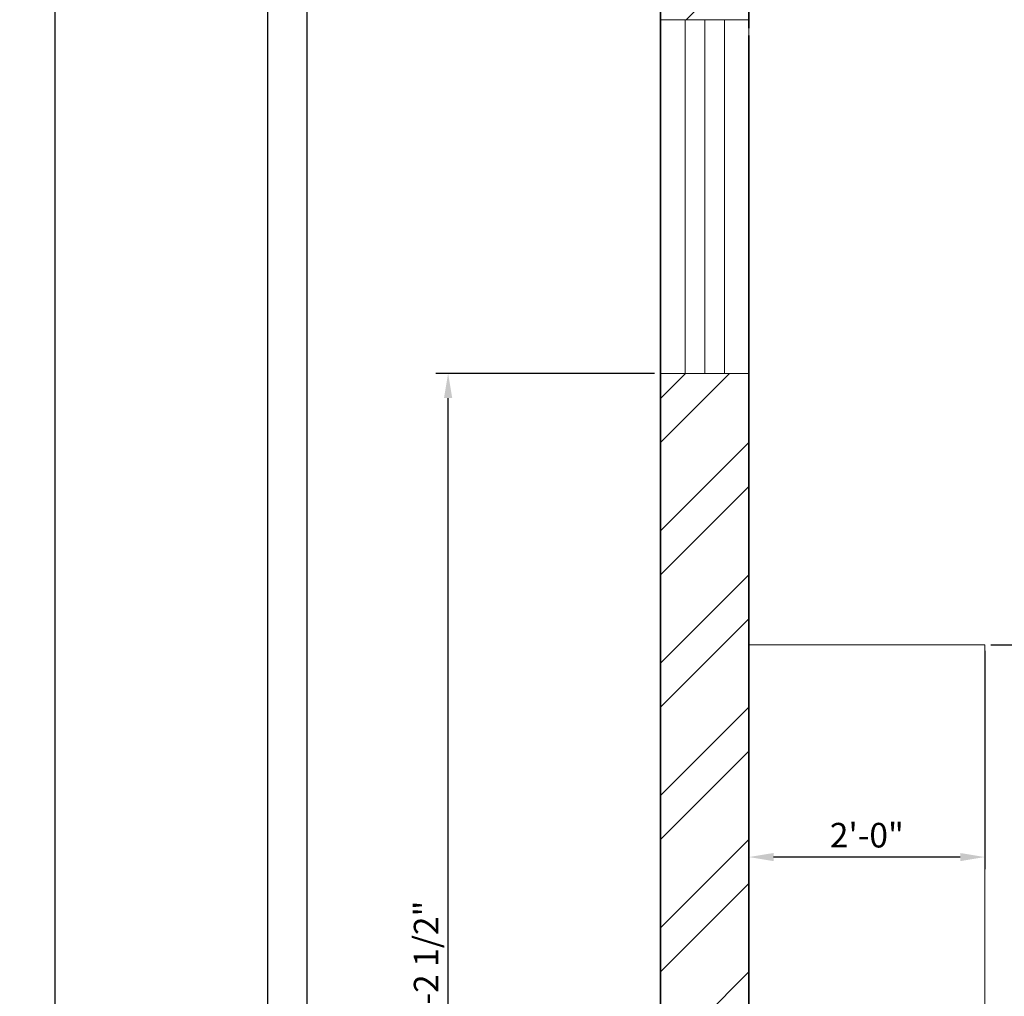
# Model space of a CAD drawing. Units: inches. Extents: x -138 to 270, y 8284 to 8764.
# Tile 2 of 10: x -138 to -38, y 8406 to 8506. Entities that reach past the tile are written whole.
import ezdxf

# ---------------------------------------------------------------- set-up
doc = ezdxf.new("R2010")
doc.units = ezdxf.units.IN
for name, color, linetype, lineweight in [('A-ANNO-DIMS', 2, 'Continuous', 18), ('A-FLOR-CASE', 9, 'Continuous', 18), ('C-PROP', 7, 'Continuous', 25), ('WALL', 8, 'Continuous', 35), ('WINDOW', 151, 'Continuous', 15)]:
    doc.layers.add(name, color=color, linetype=linetype, lineweight=lineweight)
doc.layers.add('A-WALL-PATT', color=32, linetype='Continuous', lineweight=9, true_color=0xbc761a)
doc.styles.get("Standard").update_dxf_attribs({"font": 'arial.ttf'})
doc.dimstyles.new('ISO-25', dxfattribs={"dimtxt": 2.5, "dimasz": 2.5, "dimexe": 1.25, "dimexo": 0.625, "dimtad": 1, "dimdec": 0, "dimlunit": 3, "dimtxsty": 'Standard', "dimcen": 2.5, "dimadec": 0, "dimazin": 0, "dimtfac": 1, "dimtdec": 0, "dimtmove": 0, "dimatfit": 3, "dimfxl": 1, "dimarcsym": 0})

# ---------------------------------------------------------------- blocks, each defined once
blk = doc.blocks.new('WINDOW-36IN')
for p, q in [((0, 6.5), (36, 6.5)), ((0, 4.5), (36, 4.5)), ((0, 2.5), (36, 2.5))]:
    blk.add_line(p, q)
blk.add_lwpolyline([(0, 0), (36, 0), (36, 9), (0, 9)], close=True)
blk = doc.blocks.new('*D52')
at = {"layer": 'A-ANNO-DIMS', "color": 0, "lineweight": -2, "transparency": 16777216}
for p, q in [((-113.55, 8739.24), (-135.79, 8739.24)), ((-134.54, 8309.74), (-134.54, 8736.74)), ((-113.55, 8307.24), (-135.79, 8307.24))]:
    blk.add_line(p, q, dxfattribs=at)
at = {"layer": 'A-ANNO-DIMS', "color": 0, "transparency": 16777216}
for points in [[(-134.96, 8736.74), (-134.12, 8736.74), (-134.54, 8739.24)], [(-134.96, 8309.74), (-134.12, 8309.74), (-134.54, 8307.24)]]:
    blk.add_solid(points, dxfattribs=at)
at = {"layer": 'Defpoints', "color": 0, "transparency": 16777216}
for p in [(-134.54, 8739.24), (-112.92, 8739.24), (-112.92, 8307.24)]:
    blk.add_point(p, dxfattribs=at)
at = {"layer": 'A-ANNO-DIMS', "color": 0, "transparency": 16777216, "insert": (-136.44, 8523.24), "char_height": 2.5, "attachment_point": 5, "rotation": 90}
blk.add_mtext('36\'-0"', dxfattribs=at)
blk = doc.blocks.new('*D64')
at = {"layer": 'A-ANNO-DIMS', "color": 0, "lineweight": -2, "transparency": 16777216}
for p, q in [((-73.55, 8469.84), (-95.79, 8469.84)), ((-94.54, 8349.74), (-94.54, 8467.34)), ((-73.55, 8347.24), (-95.79, 8347.24))]:
    blk.add_line(p, q, dxfattribs=at)
at = {"layer": 'A-ANNO-DIMS', "color": 0, "transparency": 16777216}
for points in [[(-94.96, 8467.34), (-94.12, 8467.34), (-94.54, 8469.84)], [(-94.96, 8349.74), (-94.12, 8349.74), (-94.54, 8347.24)]]:
    blk.add_solid(points, dxfattribs=at)
at = {"layer": 'Defpoints', "color": 0, "transparency": 16777216}
for p in [(-94.54, 8469.84), (-72.92, 8469.84), (-72.92, 8347.24)]:
    blk.add_point(p, dxfattribs=at)
at = {"layer": 'A-ANNO-DIMS', "color": 0, "transparency": 16777216, "insert": (-96.46, 8408.54), "char_height": 2.5, "attachment_point": 5, "rotation": 90}
blk.add_mtext('10\'-2 1/2"', dxfattribs=at)
blk = doc.blocks.new('*D73')
at = {"layer": 'A-ANNO-DIMS', "color": 0, "lineweight": -2, "transparency": 16777216}
for p, q in [((-63.92, 8441.62), (-63.92, 8419.38)), ((-39.92, 8441.62), (-39.92, 8419.38)), ((-42.42, 8420.63), (-61.42, 8420.63))]:
    blk.add_line(p, q, dxfattribs=at)
at = {"layer": 'A-ANNO-DIMS', "color": 0, "transparency": 16777216}
for points in [[(-61.42, 8421.04), (-61.42, 8420.21), (-63.92, 8420.63)], [(-42.42, 8421.04), (-42.42, 8420.21), (-39.92, 8420.63)]]:
    blk.add_solid(points, dxfattribs=at)
at = {"layer": 'Defpoints', "color": 0, "transparency": 16777216}
for p in [(-63.92, 8442.24), (-39.92, 8442.24), (-63.92, 8420.63)]:
    blk.add_point(p, dxfattribs=at)
at = {"layer": 'A-ANNO-DIMS', "color": 0, "transparency": 16777216, "insert": (-51.92, 8422.53), "char_height": 2.5, "attachment_point": 5}
blk.add_mtext('2\'-0"', dxfattribs=at)
blk = doc.blocks.new('*D74')
at = {"layer": 'A-ANNO-DIMS', "color": 0, "lineweight": -2, "transparency": 16777216}
for p, q in [((-39.3, 8442.24), (-17.06, 8442.24)), ((-18.31, 8439.74), (-18.31, 8382.74)), ((-39.3, 8380.24), (-17.06, 8380.24))]:
    blk.add_line(p, q, dxfattribs=at)
at = {"layer": 'A-ANNO-DIMS', "color": 0, "transparency": 16777216}
for points in [[(-18.73, 8439.74), (-17.89, 8439.74), (-18.31, 8442.24)], [(-18.73, 8382.74), (-17.89, 8382.74), (-18.31, 8380.24)]]:
    blk.add_solid(points, dxfattribs=at)
at = {"layer": 'Defpoints', "color": 0, "transparency": 16777216}
for p in [(-39.92, 8442.24), (-39.92, 8380.24), (-18.31, 8380.24)]:
    blk.add_point(p, dxfattribs=at)
at = {"layer": 'A-ANNO-DIMS', "color": 0, "transparency": 16777216, "insert": (-20.21, 8411.24), "char_height": 2.5, "attachment_point": 5, "rotation": 90}
blk.add_mtext('5\'-2"', dxfattribs=at)

msp = doc.modelspace()

# ---------------------------------------------------------------- hatches: boundary and pattern name
at = {"layer": 'A-WALL-PATT'}
h = msp.add_hatch(dxfattribs=at)
h.set_pattern_fill('ANSI32', color=256)
h.paths.add_polyline_path([(-23.4, 8356.24), (-63.92, 8356.24), (-63.92, 8347.24), (-23.4, 8347.24)])
h.paths.add_polyline_path([(-63.92, 8469.84), (-72.92, 8469.84), (-72.92, 8359.24), (-63.92, 8359.24)])
h.paths.add_polyline_path([(-63.92, 8510.27), (-72.92, 8510.27), (-72.92, 8505.84), (-63.92, 8505.84)])
h.paths.add_polyline_path([(-63.92, 8527.36), (-72.92, 8527.36), (-72.92, 8522.27), (-63.92, 8522.27)])
h.paths.add_polyline_path([(26.08, 8522.24), (24.78, 8522.24), (24.78, 8522.24), (20.08, 8522.24), (20.08, 8516.24), (-63.92, 8516.24), (-63.92, 8510.24), (26.08, 8510.24)])
h.paths.add_polyline_path([(34.02, 8398.24), (34.02, 8404.24), (26.08, 8404.24), (26.08, 8356.24), (12.6, 8356.24), (12.6, 8347.24), (37.77, 8347.24), (37.77, 8356.24), (32.08, 8356.24), (32.08, 8398.24)])
h.paths.add_polyline_path([(67.02, 8404.24), (67.02, 8398.24), (68.08, 8398.24), (68.08, 8356.24), (61.77, 8356.24), (61.77, 8347.24), (74.08, 8347.24), (74.08, 8356.24), (74.08, 8356.24), (74.08, 8449.75), (68.08, 8449.75), (68.08, 8404.24)])

# ---------------------------------------------------------------- linework, layer by layer
at = {"layer": 'A-FLOR-CASE'}
for q in [(-63.92, 8442.24), (-39.92, 8380.24)]:
    msp.add_line((-39.92, 8442.24), q, dxfattribs=at)
at = {"layer": 'C-PROP'}
for p, q in [((-112.92, 8739.24), (-112.92, 8307.24)), ((-108.92, 8735.24), (-108.92, 8311.24))]:
    msp.add_line(p, q, dxfattribs=at)
at = {"layer": 'WALL'}
for p, q in [((-63.92, 8564.99), (-63.92, 8504.99)), ((-72.92, 8528.24), (-72.92, 8347.24)), ((-63.92, 8504.24), (-63.92, 8356.24))]:
    msp.add_line(p, q, dxfattribs=at)

# ---------------------------------------------------------------- block references
at = {"layer": 'WINDOW', "extrusion": (0, 0, -1), "zscale": -1, "rotation": 89.99999999999208}
msp.add_blockref('WINDOW-36IN', (72.92, 8469.84), dxfattribs=at)

# ---------------------------------------------------------------- dimensions: what is measured, and where the dimension line sits
at = {"layer": 'A-ANNO-DIMS'}
for base, p1, p2, angle, picture, middle in [((-134.54, 8739.24), (-112.92, 8307.24), (-112.92, 8739.24), 90, '*D52', (-136.44, 8523.24)), ((-94.54, 8469.84), (-72.92, 8347.24), (-72.92, 8469.84), 90, '*D64', (-96.46, 8408.54)), ((-63.92, 8420.63), (-39.92, 8442.24), (-63.92, 8442.24), 180, '*D73', (-51.92, 8422.53)), ((-18.31, 8380.24), (-39.92, 8442.24), (-39.92, 8380.24), 270, '*D74', (-20.21, 8411.24))]:
    dim = msp.add_linear_dim(base=base, p1=p1, p2=p2, angle=angle, dimstyle='ISO-25', override={"dimdec": 1, "dimlfac": 1, "dimrnd": 0, "dimzin": 1, "dimdsep": 46, "dimlunit": 4, "dimfrac": 2}, dxfattribs=at)
    dim.commit()
    dim.dimension.update_dxf_attribs({"geometry": picture, "text_midpoint": middle})

doc.saveas('drawing.dxf')
